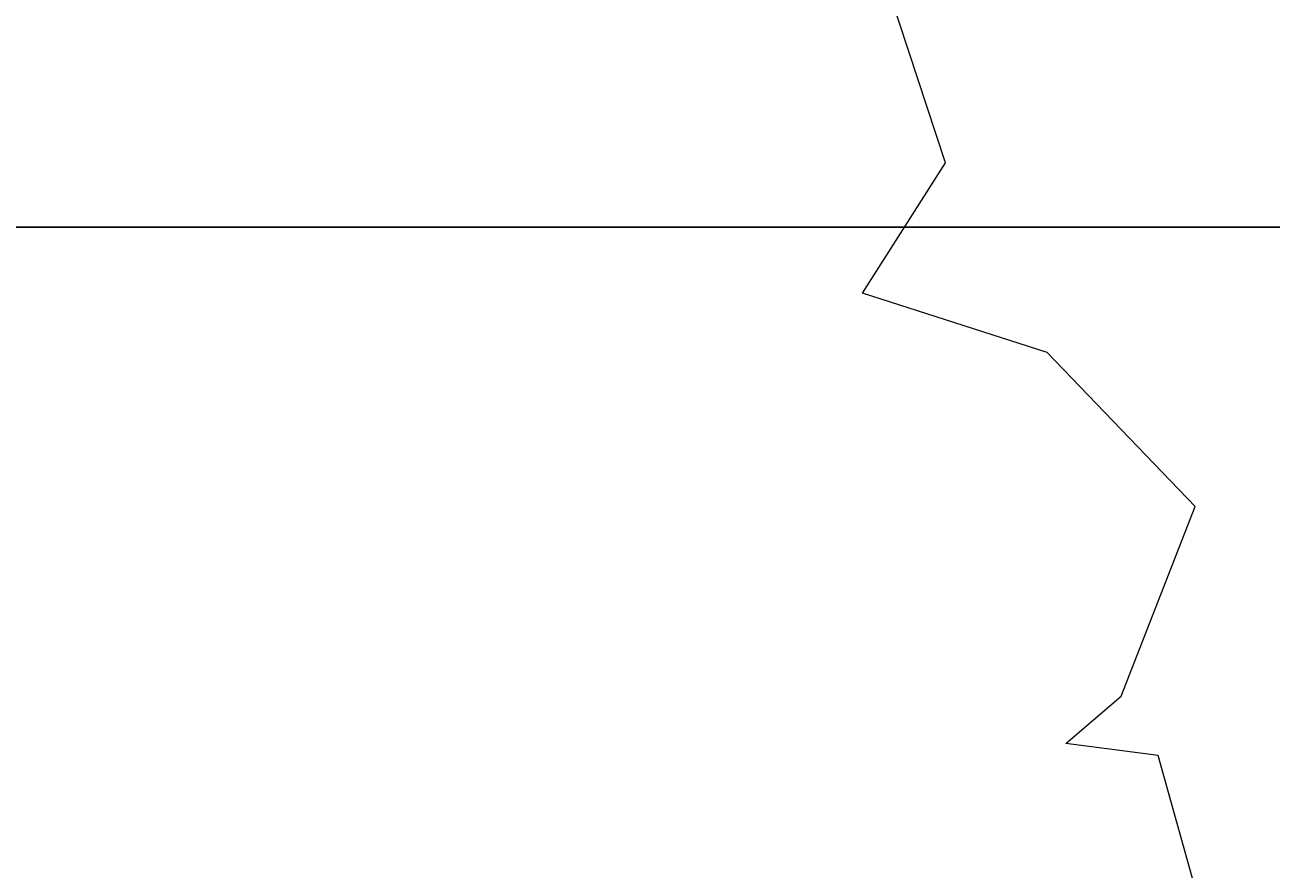
# Model space of a CAD drawing. Units: inches. Extents: x -26 to 776, y -22 to 650.
# Tile 53 of 62: x 642 to 724, y 102 to 158. Entities that reach past the tile are written whole.
import ezdxf

# ---------------------------------------------------------------- set-up
doc = ezdxf.new("R2010")
doc.units = ezdxf.units.IN
doc.header["$MEASUREMENT"] = 0
doc.layers.add('A-ANNO-DIMS', color=2, linetype='Continuous', lineweight=18)
doc.layers.add('L-PLNT-TREE', color=94, linetype='Continuous', lineweight=18)
doc.styles.get("Standard").update_dxf_attribs({"font": 'arial.ttf'})
doc.dimstyles.get("Standard").update_dxf_attribs({"dimtxt": 0.5625, "dimasz": 0.18, "dimexe": 0.18, "dimexo": 0.0625, "dimgap": 0.09, "dimtad": 0, "dimtih": 1, "dimtoh": 1, "dimdec": 4, "dimzin": 0, "dimdsep": 46, "dimlunit": 4, "dimtxsty": 'Standard', "dimcen": 0.09, "dimadec": 0, "dimazin": 0, "dimtfac": 1, "dimtdec": 4, "dimtofl": 0, "dimtmove": 0, "dimatfit": 3, "dimfxl": 1, "dimtolj": 1, "dimtzin": 0, "dimarcsym": 0})

# ---------------------------------------------------------------- blocks, each defined once
blk = doc.blocks.new('Tree - type 3 evergreen elevation')
for points in [[(56.5053, 50.874), (52.1919, 66.3574), (47.8785, 66.9103), (50.4665, 69.1222), (53.9172, 77.9699), (47.0158, 85.1586), (38.3891, 87.9235), (42.2711, 94.0063)], [(42.2711, 94.0063), (38.8204, 104.5129), (36.6637, 104.5129), (32.3503, 113.9135), (29.7623, 113.3605), (26.743, 113.3605), (24.5862, 117.7844), (25.8802, 123.8671), (29.331, 123.8671), (22.8609, 131.6088), (21.9982, 137.6916)]]:
    blk.add_lwpolyline(points)
blk = doc.blocks.new('*D20')
at = {"layer": 'A-ANNO-DIMS', "color": 0, "lineweight": -2, "transparency": 16777216}
for p, q in [((425.806, 455.472), (775.335, 455.472)), ((775.155, 455.292), (775.155, 235.854)), ((775.155, 15.662), (775.155, 235.1)), ((425.806, 15.482), (775.335, 15.482))]:
    blk.add_line(p, q, dxfattribs=at)
at = {"layer": 'A-ANNO-DIMS', "color": 0, "transparency": 16777216}
for points in [[(775.125, 455.292), (775.185, 455.292), (775.155, 455.472)], [(775.125, 15.662), (775.185, 15.662), (775.155, 15.482)]]:
    blk.add_solid(points, dxfattribs=at)
at = {"layer": 'Defpoints', "color": 0, "transparency": 16777216}
for p in [(425.743, 455.472), (775.155, 455.472), (425.743, 15.482)]:
    blk.add_point(p, dxfattribs=at)
at = {"layer": 'A-ANNO-DIMS', "color": 0, "transparency": 16777216, "insert": (775.155, 235.477), "char_height": 0.5625, "attachment_point": 5}
blk.add_mtext('\\A1;440', dxfattribs=at)
blk = doc.blocks.new('*D30')
at = {"layer": 'A-ANNO-DIMS', "color": 0, "lineweight": -2, "transparency": 16777216}
for p, q in [((280.68, 144.836), (775.335, 144.836)), ((775.155, 144.656), (775.155, 86.007)), ((775.155, 26.604), (775.155, 85.253)), ((280.68, 26.424), (775.335, 26.424))]:
    blk.add_line(p, q, dxfattribs=at)
at = {"layer": 'A-ANNO-DIMS', "color": 0, "transparency": 16777216}
for points in [[(775.125, 144.656), (775.185, 144.656), (775.155, 144.836)], [(775.125, 26.604), (775.185, 26.604), (775.155, 26.424)]]:
    blk.add_solid(points, dxfattribs=at)
at = {"layer": 'Defpoints', "color": 0, "transparency": 16777216}
for p in [(280.617, 144.836), (775.155, 144.836), (280.617, 26.424)]:
    blk.add_point(p, dxfattribs=at)
at = {"layer": 'A-ANNO-DIMS', "color": 0, "transparency": 16777216, "insert": (775.155, 85.63), "char_height": 0.5625, "attachment_point": 5}
blk.add_mtext('\\A1;118.41', dxfattribs=at)
blk = doc.blocks.new('*D45')
at = {"layer": 'A-ANNO-DIMS', "color": 0, "lineweight": -2, "transparency": 16777216}
for p, q in [((507.738, 408.639), (775.335, 408.639)), ((775.155, 408.459), (775.155, 212.438)), ((775.155, 15.662), (775.155, 211.683)), ((585.998, 15.482), (775.335, 15.482))]:
    blk.add_line(p, q, dxfattribs=at)
at = {"layer": 'A-ANNO-DIMS', "color": 0, "transparency": 16777216}
for points in [[(775.125, 408.459), (775.185, 408.459), (775.155, 408.639)], [(775.125, 15.662), (775.185, 15.662), (775.155, 15.482)]]:
    blk.add_solid(points, dxfattribs=at)
at = {"layer": 'Defpoints', "color": 0, "transparency": 16777216}
for p in [(507.676, 408.639), (775.155, 408.639), (585.935, 15.482)]:
    blk.add_point(p, dxfattribs=at)
at = {"layer": 'A-ANNO-DIMS', "color": 0, "transparency": 16777216, "insert": (775.155, 212.061), "char_height": 0.5625, "attachment_point": 5}
blk.add_mtext('\\A1;393.16', dxfattribs=at)
blk = doc.blocks.new('*D46')
at = {"layer": 'A-ANNO-DIMS', "color": 0, "lineweight": -2, "transparency": 16777216}
for p, q in [((658.506, 219.032), (775.335, 219.032)), ((775.155, 218.852), (775.155, 117.635)), ((775.155, 15.662), (775.155, 116.88)), ((677.966, 15.482), (775.335, 15.482))]:
    blk.add_line(p, q, dxfattribs=at)
at = {"layer": 'A-ANNO-DIMS', "color": 0, "transparency": 16777216}
for points in [[(775.125, 218.852), (775.185, 218.852), (775.155, 219.032)], [(775.125, 15.662), (775.185, 15.662), (775.155, 15.482)]]:
    blk.add_solid(points, dxfattribs=at)
at = {"layer": 'Defpoints', "color": 0, "transparency": 16777216}
for p in [(658.444, 219.032), (775.155, 219.032), (677.904, 15.482)]:
    blk.add_point(p, dxfattribs=at)
at = {"layer": 'A-ANNO-DIMS', "color": 0, "transparency": 16777216, "insert": (775.155, 117.257), "char_height": 0.5625, "attachment_point": 5}
blk.add_mtext('\\A1;203.55', dxfattribs=at)
blk = doc.blocks.new('*D48')
at = {"layer": 'A-ANNO-DIMS', "color": 0, "lineweight": -2, "transparency": 16777216}
for p, q in [((545.033, 67.415), (545.033, 649.856)), ((545.213, 649.676), (640.879, 649.676)), ((738.57, 649.676), (642.904, 649.676)), ((738.75, 50.911), (738.75, 649.856))]:
    blk.add_line(p, q, dxfattribs=at)
at = {"layer": 'A-ANNO-DIMS', "color": 0, "transparency": 16777216}
for points in [[(545.213, 649.706), (545.213, 649.646), (545.033, 649.676)], [(738.57, 649.706), (738.57, 649.646), (738.75, 649.676)]]:
    blk.add_solid(points, dxfattribs=at)
at = {"layer": 'Defpoints', "color": 0, "transparency": 16777216}
for p in [(738.75, 649.676), (545.033, 67.352), (738.75, 50.848)]:
    blk.add_point(p, dxfattribs=at)
at = {"layer": 'A-ANNO-DIMS', "color": 0, "transparency": 16777216, "insert": (641.892, 649.676), "char_height": 0.5625, "attachment_point": 5}
blk.add_mtext('\\A1;193.7', dxfattribs=at)

msp = doc.modelspace()

# ---------------------------------------------------------------- block references
at = {"layer": 'L-PLNT-TREE', "xscale": 1.421226385586178, "yscale": 1.421226385586178, "zscale": 1.421226385586178}
msp.add_blockref('Tree - type 3 evergreen elevation', (642.5048, 15.4824), dxfattribs=at)

# ---------------------------------------------------------------- dimensions: what is measured, and where the dimension line sits
at = {"layer": 'A-ANNO-DIMS'}
dim = msp.add_linear_dim(base=(738.7503, 649.6763), p1=(545.0331, 67.3523), p2=(738.7503, 50.8482), dimstyle='Standard', override={"dimdec": 1, "dimlfac": 1, "dimrnd": 0, "dimzin": 0, "dimdsep": 46, "dimlunit": 2}, dxfattribs=at)
dim.commit()
dim.dimension.update_dxf_attribs({"geometry": '*D48', "text_midpoint": (641.8917, 649.6763)})
for base, p1, p2, override, picture, middle in [((775.1553, 455.4717), (425.7434, 15.4824), (425.7434, 455.4717), {"dimdec": 0, "dimlfac": 1, "dimrnd": 0, "dimzin": 0, "dimdsep": 46, "dimlunit": 2}, '*D20', (775.1553, 235.477)), ((775.1553, 408.6389), (585.9354, 15.4824), (507.6759, 408.6389), {"dimdec": 2, "dimlfac": 1, "dimrnd": 0, "dimzin": 0, "dimdsep": 46, "dimlunit": 2}, '*D45', (775.1553, 212.0606)), ((775.1553, 219.0324), (677.9037, 15.4824), (658.4435, 219.0324), {"dimdec": 2, "dimlfac": 1, "dimrnd": 0, "dimzin": 0, "dimdsep": 46, "dimlunit": 2}, '*D46', (775.1553, 117.2574)), ((775.1553, 144.8359), (280.6173, 26.4239), (280.6173, 144.8359), {"dimdec": 2, "dimlfac": 1, "dimrnd": 0, "dimzin": 0, "dimdsep": 46, "dimlunit": 2}, '*D30', (775.1553, 85.6299))]:
    dim = msp.add_linear_dim(base=base, p1=p1, p2=p2, angle=90, dimstyle='Standard', override=override, dxfattribs=at)
    dim.commit()
    dim.dimension.update_dxf_attribs({"geometry": picture, "text_midpoint": middle})

doc.saveas('drawing.dxf')
